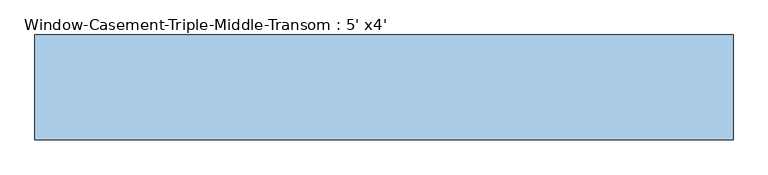
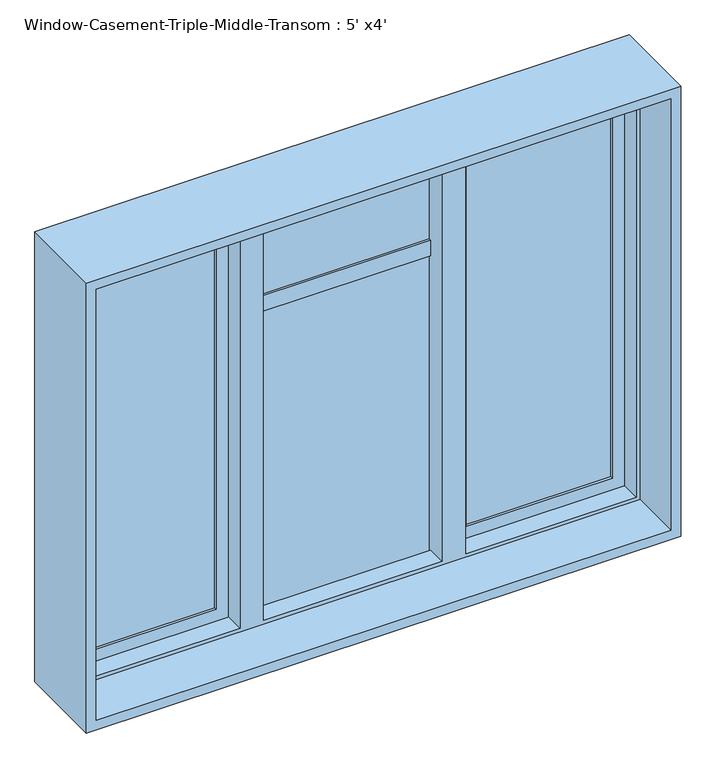
"""IFC4 building model written with IfcOpenShell, lengths in millimetres: window geometry, Window-Casement-Triple-Middle-Transom : 5' x4'."""

from ifc_helpers import new_model, si_unit, frame, origin, place, context, project, spatial, polyline, outline, extrude, faceted_brep, source, transform, mapped, element, save


def window_casement_triple_middle_transom_5_x4_de6e65d4(model_context):
    return source(origin(), model_context, "Body", "SolidModel", [
        extrude(outline(polyline([(2108.2, 279.4), (939.8, 279.4), (939.8, 736.6), (2108.2, 736.6), (2108.2, 279.4)]), holes=[polyline([(2066.3296875, 694.7296875), (981.6703125, 694.7296875), (981.6703125, 321.2703125), (2066.3296875, 321.2703125), (2066.3296875, 694.7296875)])]), frame((0.0, 73.025, 0.0), z_axis=(0.0, 1.0, 0.0), x_axis=(0.0, 0.0, 1.0)), (0.0, 0.0, 1.0), 31.75),
        extrude(outline(polyline([(2108.2, -736.6), (939.8, -736.6), (939.8, -279.4), (2108.2, -279.4), (2108.2, -736.6)]), holes=[polyline([(2066.3296875, -321.2703125), (981.6703125, -321.2703125), (981.6703125, -694.7296875), (2066.3296875, -694.7296875), (2066.3296875, -321.2703125)])]), frame((0.0, 73.025, 0.0), z_axis=(0.0, 1.0, 0.0), x_axis=(0.0, 0.0, 1.0)), (0.0, 0.0, 1.0), 31.75),
        extrude(outline(polyline([(-321.2703125, 98.425), (-321.2703125, 92.075), (-694.7296875, 92.075), (-694.7296875, 98.425), (-321.2703125, 98.425)])), frame((0.0, 0.0, 949.9203125), z_axis=(0.0, 0.0, 1.0), x_axis=(1.0, 0.0, 0.0)), (0.0, 0.0, 1.0), 1148.159375),
        extrude(outline(polyline([(-321.2703125, 85.725), (-321.2703125, 79.375), (-694.7296875, 79.375), (-694.7296875, 85.725), (-321.2703125, 85.725)])), frame((0.0, 0.0, 949.9203125), z_axis=(0.0, 0.0, 1.0), x_axis=(1.0, 0.0, 0.0)), (0.0, 0.0, 1.0), 1148.159375),
        extrude(outline(polyline([(694.7296875, 98.425), (694.7296875, 92.075), (321.2703125, 92.075), (321.2703125, 98.425), (694.7296875, 98.425)])), frame((0.0, 0.0, 949.9203125), z_axis=(0.0, 0.0, 1.0), x_axis=(1.0, 0.0, 0.0)), (0.0, 0.0, 1.0), 1148.159375),
        extrude(outline(polyline([(694.7296875, 85.725), (694.7296875, 79.375), (321.2703125, 79.375), (321.2703125, 85.725), (694.7296875, 85.725)])), frame((0.0, 0.0, 949.9203125), z_axis=(0.0, 0.0, 1.0), x_axis=(1.0, 0.0, 0.0)), (0.0, 0.0, 1.0), 1148.159375),
        extrude(outline(polyline([(228.6, 104.775), (228.6, 73.025), (-228.6, 73.025), (-228.6, 104.775), (228.6, 104.775)])), frame((0.0, 0.0, 1746.9048438), z_axis=(0.0, 0.0, 1.0), x_axis=(1.0, 0.0, 0.0)), (0.0, 0.0, 1.0), 41.8703125),
        extrude(outline(polyline([(228.6, 98.425), (228.6, 92.075), (-228.6, 92.075), (-228.6, 98.425), (228.6, 98.425)])), frame((0.0, 0.0, 939.8), z_axis=(0.0, 0.0, 1.0), x_axis=(1.0, 0.0, 0.0)), (0.0, 0.0, 1.0), 807.1048438),
        extrude(outline(polyline([(228.6, 85.725), (228.6, 79.375), (-228.6, 79.375), (-228.6, 85.725), (228.6, 85.725)])), frame((0.0, 0.0, 939.8), z_axis=(0.0, 0.0, 1.0), x_axis=(1.0, 0.0, 0.0)), (0.0, 0.0, 1.0), 807.1048438),
        extrude(outline(polyline([(228.6, 98.425), (228.6, 92.075), (-228.6, 92.075), (-228.6, 98.425), (228.6, 98.425)])), frame((0.0, 0.0, 1788.7751563), z_axis=(0.0, 0.0, 1.0), x_axis=(1.0, 0.0, 0.0)), (0.0, 0.0, 1.0), 319.4248438),
        extrude(outline(polyline([(228.6, 85.725), (228.6, 79.375), (-228.6, 79.375), (-228.6, 85.725), (228.6, 85.725)])), frame((0.0, 0.0, 1788.7751563), z_axis=(0.0, 0.0, 1.0), x_axis=(1.0, 0.0, 0.0)), (0.0, 0.0, 1.0), 319.4248438),
        faceted_brep([(-279.4, 73.025, 2108.2), (-736.6, 73.025, 2108.2), (-736.6, 114.3, 2108.2), (736.6, 114.3, 2108.2), (736.6, 73.025, 2108.2), (279.4, 73.025, 2108.2), (279.4, 111.125, 2108.2), (228.6, 111.125, 2108.2), (228.6, 73.025, 2108.2), (-228.6, 73.025, 2108.2), (-228.6, 111.125, 2108.2), (-279.4, 111.125, 2108.2), (-726.4796875, 22.225, 2098.0796875), (-726.4796875, 73.025, 2098.0796875), (-289.5203125, 73.025, 2098.0796875), (-289.5203125, 22.225, 2098.0796875), (726.4796875, 73.025, 2098.0796875), (726.4796875, 22.225, 2098.0796875), (289.5203125, 22.225, 2098.0796875), (289.5203125, 73.025, 2098.0796875), (-228.6, 73.025, 2098.0796875), (228.6, 73.025, 2098.0796875), (228.6, 22.225, 2098.0796875), (-228.6, 22.225, 2098.0796875), (-736.6, -114.3, 2108.2), (-736.6, 22.225, 2108.2), (736.6, 22.225, 2108.2), (736.6, -114.3, 2108.2), (-762.0, 114.3, 2133.6), (-762.0, -114.3, 2133.6), (762.0, -114.3, 2133.6), (762.0, 114.3, 2133.6), (736.6, 114.3, 939.8), (736.6, 73.025, 939.8), (726.4796875, 73.025, 949.9203125), (726.4796875, 22.225, 949.9203125), (736.6, 22.225, 939.8), (736.6, -114.3, 939.8), (762.0, -114.3, 914.4), (762.0, 114.3, 914.4), (279.4, 73.025, 939.8), (-736.6, 114.3, 939.8), (-736.6, 73.025, 939.8), (-279.4, 73.025, 939.8), (-279.4, 111.125, 939.8), (-228.6, 111.125, 939.8), (-228.6, 73.025, 939.8), (228.6, 73.025, 939.8), (228.6, 111.125, 939.8), (279.4, 111.125, 939.8), (289.5203125, 73.025, 949.9203125), (289.5203125, 22.225, 949.9203125), (-726.4796875, 73.025, 949.9203125), (-726.4796875, 22.225, 949.9203125), (-289.5203125, 22.225, 949.9203125), (-289.5203125, 73.025, 949.9203125), (228.6, 73.025, 949.9203125), (-228.6, 73.025, 949.9203125), (-228.6, 22.225, 949.9203125), (228.6, 22.225, 949.9203125), (-736.6, 22.225, 939.8), (-736.6, -114.3, 939.8), (-762.0, -114.3, 914.4), (-762.0, 114.3, 914.4)], [[[0, 1, 2, 3, 4, 5, 6, 7, 8, 9, 10, 11]], [[12, 13, 14, 15]], [[16, 17, 18, 19]], [[20, 21, 22, 23]], [[24, 25, 26, 27]], [[28, 29, 30, 31]], [[4, 3, 32, 33]], [[17, 16, 34, 35]], [[27, 26, 36, 37]], [[31, 30, 38, 39]], [[40, 33, 32, 41, 42, 43, 44, 45, 46, 47, 48, 49]], [[35, 34, 50, 51]], [[52, 53, 54, 55]], [[56, 57, 58, 59]], [[37, 36, 60, 61]], [[39, 38, 62, 63]], [[2, 1, 42, 41]], [[21, 20, 9, 8]], [[4, 33, 40, 5], [16, 19, 50, 34]], [[57, 56, 47, 46]], [[42, 1, 0, 43], [52, 55, 14, 13]], [[13, 12, 53, 52]], [[25, 24, 61, 60]], [[30, 29, 62, 38], [24, 27, 37, 61]], [[29, 28, 63, 62]], [[28, 31, 39, 63], [3, 2, 41, 32]], [[10, 45, 44, 11]], [[11, 44, 43, 0]], [[45, 10, 9, 20, 23, 58, 57, 46]], [[6, 49, 48, 7]], [[7, 48, 47, 56, 59, 22, 21, 8]], [[49, 6, 5, 40]], [[14, 55, 54, 15]], [[50, 19, 18, 51]], [[36, 26, 25, 60], [12, 15, 54, 53], [23, 22, 59, 58], [17, 35, 51, 18]]]),
    ])


if __name__ == "__main__":
    model = new_model("IFC4")
    model_context = context("Model", 3, world=origin())
    ifc_project = project(units=[si_unit("LENGTHUNIT", "METRE", prefix="MILLI")], contexts=[model_context])
    site = spatial("IfcSite", under=ifc_project)
    building = spatial("IfcBuilding", under=site)
    placement = place(None, origin())
    window_casement_triple_middle_transom_5_x4_shape = window_casement_triple_middle_transom_5_x4_de6e65d4(model_context)
    element("IfcWindow", 1, ObjectType="Window-Casement-Triple-Middle-Transom : 5' x4'", at=placement, inside=building, context=model_context, shape_type="MappedRepresentation", body=[
        mapped(window_casement_triple_middle_transom_5_x4_shape, transform((0.0, 0.0, 0.0), x_axis=(1.0, 0.0, 0.0), y_axis=(0.0, 1.0, 0.0), z_axis=(0.0, 0.0, 1.0))),
    ])
    save(model, "model.ifc")

# Revit data of these elements
# Type "Window-Casement-Triple-Middle-Transom : 5' x4'"
#   Type Mark = "26"
#   Fire Rating = "0.5h"
#   Assembly Code = "B2020100"
#   Analytic Construction = "Double glazing - domestic"
#   Window Width = 1' - 8"
#   Window Inset [instance default] = 0' - 0 5/8"
#   Wall Thickness [instance default] = 0' - 6"
#   Visual Light Transmittance = 0.81
#   Transom Height Ratio = 0.3
#   Thermal Resistance (R) = 1.8146 (h·ft²·°F)/BTU
#   Solar Heat Gain Coefficient = 0.76
#   Rough Width = 5' - 0 1/2"
#   Rough Height = 4' - 0 1/2"
#   Heat Transfer Coefficient (U) = 0.5511 BTU/(h·ft²·°F)
#   Height = 4' - 0"
#   Transom Height = 1' - 2.4"
#   Frame Gap 3 [instance default] = 0' - 1 83/128"
#   Frame Gap 2 [instance default] = 0' - 0 5/8"
#   Frame Gap 1 = 0' - 1 51/128"
#   Default Sill Height = 3' - 0"
#   Width = 5' - 0"
#   Frame Material = Metal - Aluminum
#   Glass Panel Material = Glass
#   Wall Closure = (empty or 0)
# Element 1 (IfcWindow, "Window-Casement-Triple-Middle-Transom : 5' x4'")
#   Wall Thickness = 0' - 9"
#   Materials on its faces: "Metal - Aluminum", "Glass"
# Materials
#   "Metal - Aluminum": class "Metal", colour RGB 247 247 247, transparency 0
#   "Glass": class "Glass", colour RGB 0 128 192, transparency 0.75, Description = "Soda Lime Glass", Cost = 0
